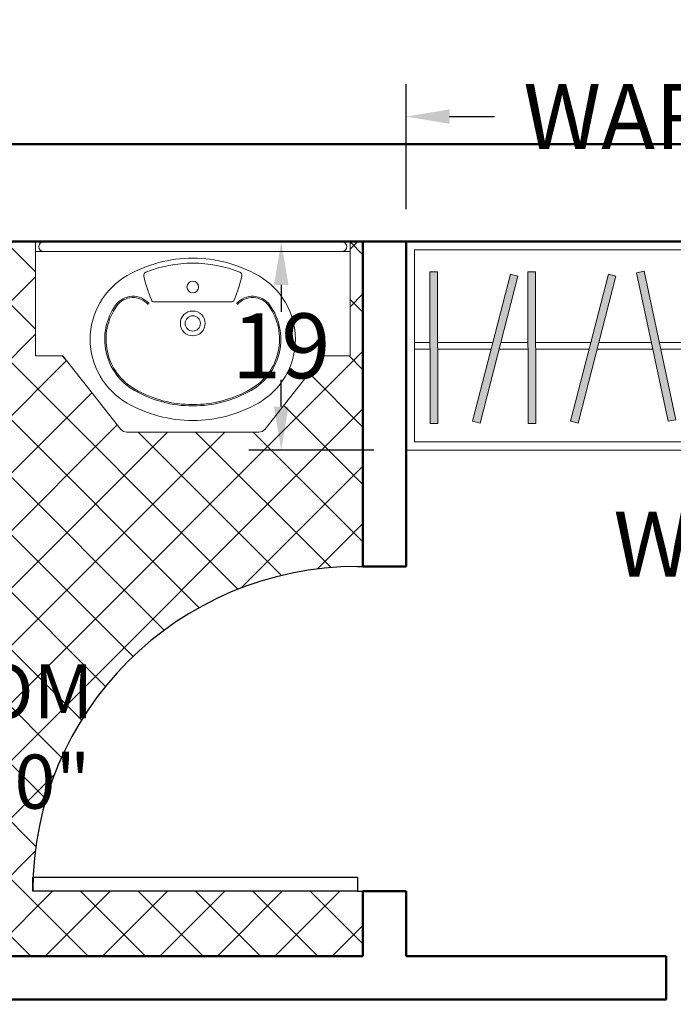
# Model space of a CAD drawing. Units: inches. Extents: x -466983 to 1020, y 324 to 318697.
# Tile 97 of 97: x 870 to 930, y 1006 to 1096. Entities that reach past the tile are written whole.
import ezdxf

# ---------------------------------------------------------------- set-up
doc = ezdxf.new("R2010")
doc.units = ezdxf.units.IN
doc.header["$MEASUREMENT"] = 0
for name, color, linetype, lineweight in [('A-ANNO-DIMS', 2, 'Continuous', 18), ('A-ANNO-TEXT', 7, 'Continuous', 18), ('A-AREA-IDEN', 7, 'Continuous', 25), ('A-DOOR', 3, 'Continuous', 25), ('A-FLOR-FIXT', 9, 'Continuous', 18), ('A-FLOR-PATT', 252, 'Continuous', 13), ('A-FURN', 8, 'Continuous', 18), ('A-WALL', 7, 'Continuous', 50)]:
    doc.layers.add(name, color=color, linetype=linetype, lineweight=lineweight)
doc.styles.get("Standard").update_dxf_attribs({"font": 'arial.ttf'})
doc.dimstyles.get("Standard").update_dxf_attribs({"dimtxt": 6, "dimasz": 4, "dimexe": 3, "dimexo": 3, "dimgap": 0.09, "dimtad": 0, "dimtih": 1, "dimtoh": 1, "dimdec": 1, "dimzin": 0, "dimdsep": 46, "dimlunit": 3, "dimtxsty": 'Standard', "dimcen": 0.09, "dimadec": 0, "dimazin": 0, "dimtfac": 1, "dimtdec": 1, "dimtofl": 0, "dimtmove": 0, "dimatfit": 3, "dimfxl": 1, "dimtolj": 1, "dimtzin": 0, "dimarcsym": 0})

# ---------------------------------------------------------------- blocks, each defined once
blk = doc.blocks.new('*U33')
for p, q in [((0, 0), (-1e-16, -5.999999999999999)), ((40, -6e-16), (40, -6))]:
    blk.add_line(p, q)
blk.add_lwpolyline([(0, 0), (5.6e-15, 40), (1.750000000000007, 40), (1.749999999999998, -7e-16)], close=True)
blk.add_arc((0, 0), 40, 0, 90)
blk = doc.blocks.new('B3')
for p, q in [((-450, 0), (-455.7402514854766, -1.1418070123309)), ((450, 0), (455.7402514854766, -1.1418070123309)), ((-463.8581929876745, -9.25974851452338), (-465, -15)), ((-465, -15), (-463.8581929876745, -20.74025148547662)), ((-460.6066017178018, -4.393398282201815), (-463.8581929876745, -9.25974851452338)), ((-463.8581929876745, -20.74025148547662), (-460.6066017178018, -25.60660171779819)), ((-455.7402514854766, -1.1418070123309), (-460.6066017178018, -4.393398282201815)), ((-460.6066017178018, -25.60660171779819), (-455.7402514854766, -28.8581929876691)), ((-455.7402514854766, -28.8581929876691), (-450, -30)), ((455.7402514854766, -28.8581929876691), (450, -30)), ((455.7402514854766, -1.1418070123309), (460.6066017177945, -4.393398282201815)), ((460.6066017177945, -25.60660171779819), (455.7402514854766, -28.8581929876691)), ((460.6066017177945, -4.393398282201815), (463.8581929876672, -9.25974851452338)), ((463.8581929876672, -20.74025148547662), (460.6066017177945, -25.60660171779819)), ((463.8581929876672, -9.25974851452338), (465, -15)), ((465, -15), (463.8581929876672, -20.74025148547662)), ((475, -30), (-475, -30)), ((2.91038e-11, -182.0000000000054), (-115.8117069986983, -182.0000000000054)), ((2.91038e-11, -182.0000000000054), (115.8117069987565, -182.0000000000054))]:
    blk.add_line(p, q)
blk.add_lwpolyline([(199.4833683843535, -575, 0.2017697719241106), (217.3542190239823, -567.482353886593), (392.5, -345), (435, -345), (475, -345), (475, 0), (-475, 0), (-475, -345), (-435, -345), (-392.5, -345), (-217.3542190239896, -567.482353886593, 0.2017697719241107), (-199.4833683843608, -575)], format="xyb", close=True)
for centre, radius, start, end in [((5.09317e-11, -450.0000000000327), 400.0000000000322, 90, 119.7172288959075), ((0, -450.0000000000327), 400.0000000000319, 60.28277110409252, 90), ((2.91038e-11, -450.0000000000055), 385, 90, 111.6513567404431), ((2.91038e-11, -450.0000000000055), 385, 68.34864325955687, 90), ((-88.47222222221171, -295.0000000000055), 221.527777777762, 119.7172288959075, 240.2827711040925), ((-138.3591766736499, -101.4576952073475), 10, 111.6513567404431, 193.3915177581575), ((338.3178096717893, 12.0282100348104), 500, 193.3915177581575, 202.0594091764406), ((-338.3178096717383, 12.0282100348104), 500, 337.9405908235594, 346.6084822418425), ((138.3591766737008, -101.4576952073475), 10, 346.6084822418425, 68.34864325955687), ((88.47222222225537, -294.9999999999964), 221.527777777762, 299.7172288959074, 60.28277110409252), ((2.91038e-11, -136.9999999999891), 17.5, 90, 270), ((2.91038e-11, -136.9999999999891), 17.5, 270, 90), ((-180.5137974189128, -229.2550553338115), 64.41699441097052, 40.71477974361456, 144.4619255202982), ((-180.5137974189128, -229.2550553338115), 60.41699441097051, 40.71477974361456, 144.4619255202982), ((-115.8117069986983, -172.0000000000145), 10, 202.0594091764406, 270), ((115.8117069987565, -172.0000000000145), 10, 270, 337.9405908235594), ((180.5137974189638, -229.2550553338115), 64.41699441097052, 35.53807447970174, 139.2852202563854), ((180.5137974189638, -229.2550553338115), 60.41699441097051, 35.53807447970174, 139.2852202563854), ((-88.47222222221171, -295.0000000000055), 177.5277777777778, 144.4619255202982, 240.2827711040925), ((-88.47222222221171, -295.0000000000055), 173.5277777777778, 144.4619255202982, 240.2827711040925), ((88.47222222223354, -295.0000000000055), 173.5277777777778, 299.7172288959074, 35.53807447970174), ((88.47222222223354, -295.0000000000055), 177.5277777777778, 299.7172288959074, 35.53807447970174), ((2.91038e-11, -247.0000000000037), 37.5, 90, 270), ((2.91038e-11, -247.0000000000037), 23, 90, 270), ((2.91038e-11, -247.0000000000037), 37.5, 270, 90), ((2.91038e-11, -247.0000000000037), 23, 270, 90), ((2.91038e-11, -140.0000000000036), 352, 240.2827711040925, 270), ((2.91038e-11, -140.0000000000036), 352, 270, 299.7172288959074), ((2.91038e-11, -140.0000000000036), 356, 240.2827711040925, 270), ((2.91038e-11, -140.0000000000036), 356, 270, 299.7172288959074), ((5.09317e-11, -139.9999999999781), 400.0000000000309, 240.2827711040925, 270), ((-1.45519e-11, -140.0000000000309), 399.9999999999781, 270, 299.7172288959074)]:
    blk.add_arc(centre, radius, start, end)
blk = doc.blocks.new('Wardrobe 1.1')
h = blk.add_hatch(color=256)
h.dxf.hatch_style = 1
h.paths.add_polyline_path([(4623.63130591675, 1559.127828082639), (4605.452274823494, 1555.618178042687), (4674.43862754123, 1198.026895294012), (4692.617658634486, 1201.536545333964)])
h = blk.add_hatch(color=256)
h.dxf.hatch_style = 1
h.paths.add_polyline_path([(4989.37316691601, 1559.911022331437), (4970.858516418657, 1559.860704815934), (4971.798831744867, 1195.677017418713), (4990.313482242336, 1195.727334934216)])
h = blk.add_hatch(color=256)
h.dxf.hatch_style = 1
h.paths.add_polyline_path([(3151.282105115228, 1187.510288244974), (3169.796885531561, 1187.510288244974), (3168.856570205235, 1551.693975642194), (3150.341919707882, 1551.643658126692)])
h = blk.add_hatch(color=256)
h.dxf.hatch_style = 1
h.paths.add_polyline_path([(3361.868584936534, 1541.669378461711), (3343.939726713163, 1546.290077294676), (3253.002619132332, 1193.641406768397), (3270.931477355587, 1189.02070793549)])
h = blk.add_hatch(color=256)
h.dxf.hatch_style = 1
h.paths.add_polyline_path([(3403.891248248334, 1551.693975642194), (3385.376597750981, 1551.643658126692), (3386.316913077191, 1187.459970729471), (3404.831563574544, 1187.510288244974)])
h = blk.add_hatch(color=256)
h.dxf.hatch_style = 1
h.paths.add_polyline_path([(3596.9032629794, 1541.669378461711), (3578.974404756262, 1546.290077294676), (3488.037297175316, 1193.641406768397), (3505.966155398454, 1189.02070793549)])
h = blk.add_hatch(color=256)
h.dxf.hatch_style = 1
h.paths.add_polyline_path([(3664.213577620618, 1553.074679382599), (3646.111361609239, 1549.18821693327), (3722.509827192224, 1193.106882382172), (3740.612043203603, 1196.993344831501)])
h = blk.add_hatch(color=256)
h.dxf.hatch_style = 1
h.paths.add_polyline_path([(3813.833679657712, 1190.320201264565), (3832.296488257873, 1188.934736184298), (3859.597907476409, 1552.094859088468), (3841.135098876248, 1553.480324168735)])
h = blk.add_hatch(color=256)
h.dxf.hatch_style = 1
h.paths.add_polyline_path([(4029.392729275909, 1551.693975642194), (4010.878078778556, 1551.643658126692), (4011.818394104767, 1187.459970729471), (4030.333044602236, 1187.510288244974)])
h = blk.add_hatch(color=256)
h.dxf.hatch_style = 1
h.paths.add_polyline_path([(4222.404744007092, 1541.669378461711), (4204.475885783836, 1546.290077294676), (4113.538778203007, 1193.641406768397), (4131.467636426145, 1189.02070793549)])
h = blk.add_hatch(color=256)
h.dxf.hatch_style = 1
h.paths.add_polyline_path([(4348.011308219915, 1193.106882382172), (4366.113524231294, 1196.993344831501), (4289.715058648309, 1553.074679382599), (4271.612842636931, 1549.18821693327)])
h = blk.add_hatch(color=256)
h.dxf.hatch_style = 1
h.paths.add_polyline_path([(4837.600952654661, 1550.260731044678), (4819.316543353771, 1553.17194924514), (4762.004005428219, 1193.525017719703), (4780.288414729109, 1190.613799519242)])
h = blk.add_hatch(color=256)
h.dxf.hatch_style = 1
h.paths.add_polyline_path([(4895.873954488479, 1554.659198605851), (4877.410424046501, 1553.283386659738), (4902.671188982951, 1196.772307061869), (4921.13471942493, 1198.148119007923)])
at = {"ltscale": 5}
for p, q in [((3093.82979383441, 1124.111993690416), (3093.82979383441, 1624.111993690416)), ((3093.82979383441, 1624.111993690416), (5093.829793834409, 1624.111993690416)), ((5093.829793834409, 1624.111993690416), (5093.829793834409, 1124.111993690416)), ((5093.829793834409, 1124.111993690416), (3093.82979383441, 1124.111993690416))]:
    blk.add_line(p, q, dxfattribs=at)
for p, q in [((3113.82979383441, 1144.111993690416), (3113.82979383441, 1604.111993690416)), ((3113.82979383441, 1604.111993690416), (5073.829793834409, 1604.111993690416)), ((5073.829793834409, 1604.111993690416), (5073.829793834409, 1144.111993690416)), ((4623.63130591675, 1559.127828082639), (4605.452274823494, 1555.618178042687)), ((4692.617658634486, 1201.536545333964), (4623.63130591675, 1559.127828082639)), ((4989.37316691601, 1559.911022331437), (4970.858516418657, 1559.860704815934)), ((4970.858516418657, 1559.860704815934), (4971.798831744867, 1195.677017418713)), ((4990.313482242336, 1195.727334934216), (4989.37316691601, 1559.911022331437)), ((3168.856570205235, 1551.693975642194), (3150.341919707882, 1551.643658126692)), ((3150.341919707882, 1551.643658126692), (3151.282235034092, 1187.459970729471)), ((3169.796885531561, 1187.510288244974), (3168.856570205235, 1551.693975642194)), ((3343.939726713163, 1546.290077294676), (3253.002619132332, 1193.641406768397)), ((3270.931477355587, 1189.02070793549), (3361.868584936534, 1541.669378461711)), ((3361.868584936534, 1541.669378461711), (3343.939726713163, 1546.290077294676)), ((3403.891248248334, 1551.693975642194), (3385.376597750981, 1551.643658126692)), ((3385.376597750981, 1551.643658126692), (3386.316913077191, 1187.459970729471)), ((3404.831563574544, 1187.510288244974), (3403.891248248334, 1551.693975642194)), ((3578.974404756262, 1546.290077294676), (3488.037297175316, 1193.641406768397)), ((3505.966155398454, 1189.02070793549), (3596.9032629794, 1541.669378461711)), ((3596.9032629794, 1541.669378461711), (3578.974404756262, 1546.290077294676)), ((3664.213577620618, 1553.074679382599), (3646.111361609239, 1549.18821693327)), ((3646.111361609239, 1549.18821693327), (3722.509827192224, 1193.106882382172)), ((3740.612043203603, 1196.993344831501), (3664.213577620618, 1553.074679382599)), ((3841.135098876248, 1553.480324168735), (3813.833679657712, 1190.320201264565)), ((3832.296488257873, 1188.934736184298), (3859.597907476409, 1552.094859088468)), ((3859.597907476409, 1552.094859088468), (3841.135098876248, 1553.480324168735)), ((4029.392729275909, 1551.693975642194), (4010.878078778556, 1551.643658126692)), ((4010.878078778556, 1551.643658126692), (4011.818394104767, 1187.459970729471)), ((4030.333044602236, 1187.510288244974), (4029.392729275909, 1551.693975642194)), ((4204.475885783836, 1546.290077294676), (4113.538778203007, 1193.641406768397)), ((4131.467636426145, 1189.02070793549), (4222.404744007092, 1541.669378461711)), ((4222.404744007092, 1541.669378461711), (4204.475885783836, 1546.290077294676)), ((4289.715058648309, 1553.074679382599), (4271.612842636931, 1549.18821693327)), ((4271.612842636931, 1549.18821693327), (4348.011308219915, 1193.106882382172)), ((4366.113524231294, 1196.993344831501), (4289.715058648309, 1553.074679382599)), ((4605.452274823494, 1555.618178042687), (4674.43862754123, 1198.026895294012)), ((4819.316543353771, 1553.17194924514), (4762.004005428219, 1193.525017719703)), ((4780.288414729109, 1190.613799519242), (4837.600952654661, 1550.260731044678)), ((4837.600952654661, 1550.260731044678), (4819.316543353771, 1553.17194924514)), ((4895.873954488479, 1554.659198605851), (4877.410424046501, 1553.283386659738)), ((4877.410424046501, 1553.283386659738), (4902.671188982951, 1196.772307061869)), ((4921.13471942493, 1198.148119007923), (4895.873954488479, 1554.659198605851)), ((3150.779647227988, 1382.111993690416), (3113.82979383441, 1382.111993690416)), ((3301.603312885615, 1382.111993690416), (3169.294427644258, 1382.111993690416)), ((3301.603312885671, 1382.111993690416), (3169.294427644278, 1382.111993690416)), ((3385.814325271087, 1382.111993690416), (3320.723705409183, 1382.111993690416)), ((3536.63799092866, 1382.111993690416), (3404.329105687303, 1382.111993690416)), ((3536.637990928537, 1382.111993690416), (3404.329105687377, 1382.111993690416)), ((3681.958135513426, 1382.111993690416), (3555.75838345205, 1382.111993690416)), ((3681.958135513406, 1382.111993690416), (3555.758383452127, 1382.111993690416)), ((3828.252080240405, 1382.111993690416), (3700.894205307252, 1382.111993690416)), ((3828.252080240453, 1382.111993690416), (3700.894205307288, 1382.111993690416)), ((4011.315806298681, 1382.111993690416), (3846.819044447374, 1382.111993690416)), ((4162.139471956229, 1382.111993690416), (4029.830586714952, 1382.111993690416)), ((4307.459616541096, 1382.111993690416), (4181.259864479818, 1382.111993690416)), ((4453.753561268143, 1382.111993690416), (4326.395686334979, 1382.111993690416)), ((4638.925011464094, 1382.111993690416), (4472.320525475011, 1382.111993690416)), ((4792.056807955193, 1382.111993690416), (4657.781122696752, 1382.111993690416)), ((4889.538855865531, 1382.111993690416), (4810.805142536459, 1382.111993690416)), ((4971.317460196375, 1382.111993690416), (4908.099870128257, 1382.111993690416)), ((5073.829793834409, 1382.111993690416), (4989.832240612645, 1382.111993690416)), ((3150.820958922443, 1366.111993690417), (3113.82979383441, 1366.111993690416)), ((3297.477411264826, 1366.111993690417), (3169.335739338719, 1366.111993690417)), ((3297.477411264836, 1366.111993690416), (3169.33573933882, 1366.111993690416)), ((3385.855636965543, 1366.111993690416), (3316.597803788389, 1366.111993690416)), ((3532.512089307866, 1366.111993690416), (3404.370417381759, 1366.111993690416)), ((3532.512089307935, 1366.111993690416), (3404.370417381687, 1366.111993690416)), ((3685.390990119154, 1366.111993690416), (3551.632481831255, 1366.111993690417)), ((3685.390990119244, 1366.111993690416), (3551.632481831408, 1366.111993690416)), ((3827.049242483872, 1366.111993690416), (3704.32705991298, 1366.111993690416)), ((3827.049242483967, 1366.111993690416), (3704.327059913011, 1366.111993690416)), ((4011.357117993108, 1366.111993690416), (3845.61620669084, 1366.111993690416)), ((4158.013570335509, 1366.111993690416), (4029.871898409377, 1366.111993690416)), ((4310.892471146819, 1366.111993690416), (4177.133962858983, 1366.111993690416)), ((4452.550723511541, 1366.111993690416), (4329.828540940702, 1366.111993690416)), ((4642.011724414702, 1366.111993690416), (4471.117687718526, 1366.111993690416)), ((4789.507083415918, 1366.111993690416), (4660.867835647359, 1366.111993690416)), ((4890.672543602346, 1366.111993690416), (4808.255417997067, 1366.111993690416)), ((4971.3587718908, 1366.111993690416), (4909.233557865072, 1366.111993690416)), ((5073.829793834409, 1366.111993690416), (4989.873552307186, 1366.111993690416)), ((3169.796885531561, 1187.510288244974), (3151.282105115229, 1187.510288244974)), ((3253.002619132332, 1193.641406768397), (3270.931477355587, 1189.02070793549)), ((3404.831563574544, 1187.510288244974), (3386.316913077191, 1187.459970729471)), ((3488.037297175316, 1193.641406768397), (3505.966155398454, 1189.02070793549)), ((3722.509827192224, 1193.106882382172), (3740.612043203603, 1196.993344831501)), ((3832.296488257873, 1188.934736184298), (3813.833679657712, 1190.320201264565)), ((4030.333044602236, 1187.510288244974), (4011.818394104767, 1187.459970729471)), ((4113.538778203007, 1193.641406768397), (4131.467636426145, 1189.02070793549)), ((4348.011308219915, 1193.106882382172), (4366.113524231294, 1196.993344831501)), ((4674.43862754123, 1198.026895294012), (4692.617658634486, 1201.536545333964)), ((4762.004005428219, 1193.525017719703), (4780.288414729109, 1190.613799519242)), ((4902.671188982951, 1196.772307061869), (4921.13471942493, 1198.148119007923)), ((4971.798831744867, 1195.677017418713), (4990.313482242336, 1195.727334934216)), ((5073.829793834409, 1144.111993690416), (3113.82979383441, 1144.111993690416))]:
    blk.add_line(p, q)
blk.add_lwpolyline([(4439.335160685403, 1190.320201264565), (4466.63657990394, 1553.480324168735), (4485.0993885041, 1552.094859088468), (4457.797969285564, 1188.934736184298), (4439.231005078596, 1188.934736184298)])
blk = doc.blocks.new('*D85')
at = {"layer": 'A-ANNO-DIMS', "color": 0, "lineweight": -2, "transparency": 16777216}
for p, q in [((905.8056775209042, 1078.937732818421), (905.8056775209042, 1090.487732818421)), ((982.805677520904, 1078.937732818421), (982.805677520904, 1090.487732818421)), ((909.805677520904, 1087.487732818421), (913.9496475072615, 1087.487732818421)), ((978.805677520904, 1087.487732818421), (974.6617075345467, 1087.487732818421))]:
    blk.add_line(p, q, dxfattribs=at)
at = {"layer": 'A-ANNO-DIMS', "color": 0, "transparency": 16777216}
for points in [[(909.805677520904, 1088.154399485087), (909.805677520904, 1086.821066151754), (905.8056775209042, 1087.487732818421)], [(978.805677520904, 1088.154399485087), (978.805677520904, 1086.821066151754), (982.805677520904, 1087.487732818421)]]:
    blk.add_solid(points, dxfattribs=at)
at = {"layer": 'Defpoints', "color": 0, "transparency": 16777216}
for p in [(982.805677520904, 1087.487732818421), (905.8056775209042, 1075.937732818421), (982.805677520904, 1075.937732818421)]:
    blk.add_point(p, dxfattribs=at)
at = {"layer": 'A-ANNO-DIMS', "color": 0, "transparency": 16777216, "insert": (944.305677520904, 1087.487732818421), "char_height": 6, "attachment_point": 5}
blk.add_mtext('\\A1;WARDROBE 77', dxfattribs=at)
blk = doc.blocks.new('*D86')
at = {"layer": 'A-ANNO-DIMS', "color": 0, "lineweight": -2, "transparency": 16777216}
for p, q in [((902.8056775209046, 1075.937732818421), (891.2556775209051, 1075.937732818421)), ((894.2556775209052, 1071.937732818421), (894.2556775209052, 1069.466170744751)), ((894.2556775209052, 1060.687732818421), (894.2556775209052, 1063.159294892091)), ((902.8056775209046, 1056.687732818421), (891.2556775209051, 1056.687732818421))]:
    blk.add_line(p, q, dxfattribs=at)
at = {"layer": 'A-ANNO-DIMS', "color": 0, "transparency": 16777216}
for points in [[(893.5890108542384, 1071.937732818421), (894.9223441875718, 1071.937732818421), (894.2556775209052, 1075.937732818421)], [(893.5890108542384, 1060.687732818421), (894.9223441875718, 1060.687732818421), (894.2556775209052, 1056.687732818421)]]:
    blk.add_solid(points, dxfattribs=at)
at = {"layer": 'Defpoints', "color": 0, "transparency": 16777216}
for p in [(894.2556775209052, 1075.937732818421), (905.8056775209045, 1075.937732818421), (905.8056775209045, 1056.687732818421)]:
    blk.add_point(p, dxfattribs=at)
at = {"layer": 'A-ANNO-DIMS', "color": 0, "transparency": 16777216, "insert": (894.2556775209052, 1066.312732818421), "char_height": 6, "attachment_point": 5}
blk.add_mtext('\\A1;19', dxfattribs=at)

msp = doc.modelspace()

# ---------------------------------------------------------------- hatches: boundary and pattern name
at = {"layer": 'A-FLOR-PATT', "transparency": 33554572}
h = msp.add_hatch(dxfattribs=at)
h.set_pattern_fill('ANSI37', color=256, scale=30)
h.set_pattern_definition([(45, (-1212.413693079869, -290.0350025265127), (-2.651650429449553, 2.651650429449553), []), (135, (-1212.413693079869, -290.0350025265127), (-2.651650429449553, -2.651650429449552), [])])
h.paths.add_polyline_path([(901.805677520904, 1075.937732818422), (900.6144036774049, 1075.937732818422), (900.6144036774049, 1065.385628316983), (899.390971271441, 1065.385628316983), (898.0910743401043, 1065.385628316983), (892.8355944880973, 1058.709752245277, -0.2583770168556315), (892.18750428989, 1058.350891982691), (879.9847834232776, 1058.350891982691, -0.2017697719240963), (879.438188978411, 1058.580825279484), (874.0812133730635, 1065.385628316983), (872.7813164417267, 1065.385628316983), (871.5578840357629, 1065.385628316983), (871.5578840357629, 1075.937732818422), (813.8056775209042, 1075.937732818422), (813.8056775209042, 1044.792233318721), (832.3947444543938, 1044.792233318721, -0.3947951267487684), (848.6601780212009, 1028.535584015862), (848.6601780212009, 1009.937732818421), (901.805677520904, 1009.937732818421), (901.805677520904, 1015.937732818421), (901.3056775209042, 1015.937732818421), (871.3056775209039, 1015.937732818421), (871.3056775209039, 1017.250232818421), (871.3344022102003, 1017.250232818421, -0.4014527144963572), (901.3056775209042, 1045.937732818421), (901.805677520904, 1045.937732818421)])
edge = h.paths.add_edge_path(flags=16)
edge.add_line((847.7730719745084, 1068.948588737025), (847.7730719745069, 1073.708823774771))
edge.add_arc((849.2268986539951, 1073.708823774771), 1.453826679487974, 90, 180, ccw=False)
edge.add_line((849.2268986539951, 1075.162650454259), (864.4920787886183, 1075.162650454259))
edge.add_arc((864.4920787886213, 1073.708823774771), 1.453826679487974, 0, 90.00000000012102, ccw=False)
edge.add_line((865.9459054681093, 1073.708823774771), (865.9459054681081, 1069.00351244647))
edge.add_arc((832.6447385074767, 1068.976050591752), 33.30117828385809, -20.61233806670998, 0.04724903539101888, ccw=False)
edge.add_ellipse((856.8594887213083, 1058.479989307073), major_axis=(-2.091e-13, 10.21313242340307), ratio=0.6859192225533502, start_angle=100.00884331843292, end_angle=259.9911566815624, ccw=False)
edge.add_arc((881.0742389351396, 1068.976050591752), 33.30117828385809, 180.0472490354062, 200.6123380667097, ccw=False)
h.paths.add_polyline_path([(853.145578187156, 1066.481532374271), (853.145578187156, 1066.453444752512), (853.1463399851561, 1066.453444752512, 0.4331071439582673), (852.9166149812349, 1066.684892837266), (852.9166149812349, 1066.453444752512), (853.145578187156, 1066.453444752512), (853.145578187156, 1066.481532374489), (853.088019486549, 1066.612171966583, 0.6979386910037918), (852.699540939094, 1066.453444752512), (852.7003027371272, 1066.453444752512), (852.7003027371272, 1066.481532374489), (852.9166149812349, 1067.001204630995), (852.9166149812349, 1066.684892837266, -0.3962543063594317)], flags=0)
h.paths.add_polyline_path([(861.0186747055222, 1066.481532374271), (861.0186747055222, 1066.453444752512), (861.0194365035225, 1066.453444752512, 0.4164039232557909), (860.8023624614146, 1066.684892837265), (860.8023624614146, 1066.453444752512), (861.0186747055222, 1066.453444752512), (861.0186747055222, 1066.481532374489), (860.9671752720659, 1066.605255499379, 0.7133437187663149), (860.5726374574602, 1066.453444752512), (860.5733992554934, 1066.453444752512), (860.5733992554934, 1066.481532374489), (860.8023624614146, 1067.001204630995), (860.8023624614146, 1066.684892837265, -0.3799725304814568)], flags=0)
edge = h.paths.add_edge_path(flags=0)
edge.add_spline(control_points=[(861.1298377106021, 1065.785468371534), (861.4660965533383, 1065.247811229462), (861.613385559155, 1065.016139861057), (861.9832837951076, 1064.373617117607), (862.1924105327118, 1063.944313665492), (862.5613774174725, 1063.039129539609), (862.7212131906668, 1062.56326642291), (862.9865156700853, 1061.578122280975), (863.0919804897928, 1061.068856600952), (863.2452407883674, 1060.031049745086), (863.293035446714, 1059.502522766744), (863.3294736797056, 1058.440879580113), (863.3181170778639, 1057.907777155726), (863.2366033468288, 1056.85179603536), (863.1664466211855, 1056.328931215311), (862.9695120306455, 1055.307951977375), (862.8427353108815, 1054.809852090196), (862.5365466723708, 1053.852219447362), (862.3571373353129, 1053.392702749349), (861.9514237071658, 1052.524888245794), (861.7251255454219, 1052.116609101398), (861.2330086320977, 1051.362239687588), (860.9672044472572, 1051.016170456457), (860.4047960485765, 1050.394909316517), (860.1082220871676, 1050.119734477926), (859.493696255806, 1049.64606200509), (859.1757900615103, 1049.447558762665), (858.5275631429041, 1049.129883644436), (858.197273503909, 1049.010664382187), (857.5314773710529, 1048.851811036626), (857.1959384637446, 1048.812116564677), (856.5249326641573, 1048.811967422545), (856.1893892160524, 1048.851512676201), (855.5235728169741, 1049.010066967686), (855.1932673158994, 1049.129136347874), (854.5449932971788, 1049.446513839261), (854.2270557868354, 1049.644869411481), (853.6124495619564, 1050.118254324803), (853.3158265363004, 1050.393289340464), (852.7533025914207, 1051.014284587242), (852.487431959371, 1051.360227769297), (851.9951668313728, 1052.114363776776), (851.7687869247744, 1052.522535562859), (851.3628973914427, 1053.390157753425), (851.1833939042357, 1053.849589492002), (850.8770077813263, 1054.807077270704), (850.7501277313783, 1055.30511724975), (850.5529806633081, 1056.326003473117), (850.4827147921034, 1056.848835185142), (850.4009803807432, 1057.904777820697), (850.3895122452288, 1058.437874867502), (850.425728471152, 1059.499535178563), (850.4734126571939, 1060.02808465918), (850.6264565107679, 1061.065963770327), (850.7318153592672, 1061.575279204679), (850.9969137893603, 1062.560548677974), (851.1566514873134, 1063.036487374614), (851.525433403113, 1063.94184619004), (851.7344732542367, 1064.371248757046), (852.1056260411488, 1065.016350037675), (852.2544071072941, 1065.250281998093), (852.608154630964, 1065.733465727338)], knot_values=[3.915332106759953, 3.915332106759953, 3.915332106759953, 3.915332106759953, 4.013467662305501, 4.013467662305501, 4.175531746215815, 4.175531746215815, 4.337595830126129, 4.337595830126129, 4.499659914036444, 4.499659914036444, 4.661723997946757, 4.661723997946757, 4.82378808185707, 4.82378808185707, 4.985852165767384, 4.985852165767384, 5.147916249677697, 5.147916249677697, 5.30998033358801, 5.30998033358801, 5.472044417498324, 5.472044417498324, 5.634108501408637, 5.634108501408637, 5.79617258531895, 5.79617258531895, 5.958236669229264, 5.958236669229264, 6.120300753139577, 6.120300753139577, 6.282364837049891, 6.282364837049891, 6.444428920960204, 6.444428920960204, 6.606493004870517, 6.606493004870517, 6.768557088780831, 6.768557088780831, 6.930621172691144, 6.930621172691144, 7.092685256601457, 7.092685256601457, 7.254749340511771, 7.254749340511771, 7.416813424422084, 7.416813424422084, 7.578877508332397, 7.578877508332397, 7.740941592242711, 7.740941592242711, 7.903005676153024, 7.903005676153024, 8.065069760063338, 8.065069760063338, 8.22713384397365, 8.22713384397365, 8.389197927883965, 8.389197927883965, 8.551262011794279, 8.551262011794279, 8.650370494357087, 8.650370494357087, 8.650370494357087, 8.650370494357087], degree=3, periodic=0)
edge.add_line((852.6421178657537, 1065.785468371534), (861.1298377106024, 1065.785468371534))
edge = h.paths.add_edge_path(flags=0)
edge.add_ellipse((856.8495804607978, 1057.743205248224), major_axis=(-3.1e-13, 7.792134415209829), ratio=0.6878610933899516, start_angle=0, end_angle=360)
h.paths.add_polyline_path([(848.8634419841151, 1069.389059844444), (848.863441984139, 1073.960453158315, -0.4142135623709757), (849.9538119937549, 1075.050823167924), (863.765165448898, 1075.050823167924, -0.4142135623721942), (864.8555354585106, 1073.960453158308), (864.8555354584933, 1069.389059844444, -0.3889362887010341), (864.5236837164459, 1069.026979909221, -0.0435607626104464), (849.19529372618, 1069.02697990933, -0.3889362886276668)], flags=0)
h.paths.add_polyline_path([(853.1006153779753, 1068.112209480768, -1), (852.677499999749, 1068.112209480768, -1)], flags=0)
edge = h.paths.add_edge_path(flags=0)
edge.add_ellipse((856.8594887213083, 1057.33782914961), major_axis=(7.74e-14, 2.20702192546696), ratio=0.6571642650458812, start_angle=0, end_angle=360)
h.paths.add_polyline_path([(861.0414774428674, 1068.112209480768, -1), (860.6183620646412, 1068.112209480768, -1)], flags=0)
edge = h.paths.add_edge_path()
edge.add_line((573.9536545579417, 1057.341203598636), (573.9536545579417, 1075.937732818422))
edge.add_line((573.9536545579417, 1075.937732818422), (558.7307922536265, 1075.937732818422))
edge.add_line((558.7307922536265, 1075.937732818422), (558.7307922536265, 1065.385628316983))
edge.add_line((558.7307922536265, 1065.385628316983), (557.5073598476627, 1065.385628316983))
edge.add_line((557.5073598476627, 1065.385628316983), (556.207462916326, 1065.385628316983))
edge.add_line((556.207462916326, 1065.385628316983), (550.9519830643189, 1058.709752245277))
edge.add_arc((550.3038928661116, 1059.115537236419), 0.7646452537275144, 270, 327.94831933647396, ccw=False)
edge.add_line((550.3038928661116, 1058.350891982691), (538.1011719994992, 1058.350891982691))
edge.add_arc((538.1011719994992, 1059.115537236419), 0.7646452537275137, 224.3704013916024, 270, ccw=False)
edge.add_line((537.5545775546327, 1058.580825279484), (532.1976019492852, 1065.385628316983))
edge.add_line((532.1976019492852, 1065.385628316983), (530.8977050179485, 1065.385628316983))
edge.add_line((530.8977050179485, 1065.385628316983), (529.6742726119846, 1065.385628316983))
edge.add_line((529.6742726119846, 1065.385628316983), (529.6742726119846, 1075.937732818422))
edge.add_line((529.6742726119846, 1075.937732818422), (520.8056775209042, 1075.937732818422))
edge.add_line((520.8056775209042, 1075.937732818422), (520.8056775209042, 1045.937732818422))
edge.add_line((520.8056775209042, 1045.937732818422), (521.3056775209044, 1045.937732818422))
edge.add_arc((521.3056775209042, 1015.937732818422), 30.00000000000023, 2.507490703587223, 89.99999999999977, ccw=False)
edge.add_line((551.2769528316082, 1017.250232818422), (551.3056775209045, 1017.250232818422))
edge.add_line((551.3056775209045, 1017.250232818422), (551.3056775209045, 1015.937732818422))
edge.add_line((551.3056775209045, 1015.937732818422), (520.8056775209042, 1015.937732818422))
edge.add_line((520.8056775209042, 1015.937732818422), (520.8056775209042, 1009.937732818421))
edge.add_line((520.8056775209042, 1009.937732818421), (559.1912990237018, 1010.402158339383))
edge.add_arc((559.1912990237018, 1011.855985018871), 1.453826679487974, 180, 270, ccw=False)
edge.add_line((557.7374723442138, 1011.855985018871), (557.7374723442151, 1016.561296347171))
edge.add_arc((591.0386393048469, 1016.58875820189), 33.3011782838587, 159.3876619332891, 180.0472490353913, ccw=False)
edge.add_ellipse((566.8238890910148, 1027.084819486569), major_axis=(-3.171e-13, 10.21313242340307), ratio=0.6859192225533445, start_angle=280.00884331843395, end_angle=439.99115668156304, ccw=False)
edge.add_arc((542.6091388771833, 1016.58875820189), 33.3011782838584, 0.04724903544490644, 20.612338066710322, ccw=False)
edge.add_line((575.9103058378148, 1016.61622005664), (575.910305837816, 1011.855985018871))
edge.add_arc((574.4564791583282, 1011.855985018871), 1.453826679487974, -90, 0, ccw=False)
edge.add_line((574.4564791583282, 1010.402158339383), (608.8056775209044, 1009.937732818421))
edge.add_line((608.8056775209044, 1009.937732818421), (608.8056775209044, 1041.08570985546))
edge.add_line((608.8056775209044, 1041.08570985546), (590.2179319406538, 1041.08570985546))
edge.add_arc((590.7750219589672, 1057.907380652626), 16.83089295601249, 181.9277454211679, 268.1032059320871, ccw=False)
edge = h.paths.add_edge_path()
edge.add_ellipse((494.2443328575609, 583.6203939656394), major_axis=(-2.099e-13, 10.21313242340307), ratio=0.6859192225533391, start_angle=280.0088433184392, end_angle=439.99115668155895, ccw=False)
edge.add_arc((470.0295826437295, 573.1243326809605), 33.30117828385828, 0.047249035653180727, 20.612338066711573, ccw=False)
edge.add_line((503.3307496043607, 573.1517945358311), (503.3307496043621, 568.3915594979414))
edge.add_arc((501.8769229248741, 568.3915594979414), 1.453826679487974, -90, 0, ccw=False)
edge.add_line((501.8769229248741, 566.9377328184536), (539.8056775209043, 566.9377328184218))
edge.add_line((539.8056775209043, 566.9377328184218), (539.8056775209043, 572.9377328184218))
edge.add_line((539.8056775209043, 572.9377328184218), (539.3056775209043, 572.9377328184218))
edge.add_line((539.3056775209043, 572.9377328184218), (509.3056775209042, 572.9377328184218))
edge.add_line((509.3056775209042, 572.9377328184218), (509.3056775209042, 574.2502328184218))
edge.add_line((509.3056775209042, 574.2502328184218), (509.3344022102004, 574.2502328184218))
edge.add_arc((539.3056775209043, 572.9377328184218), 30.00000000000003, 90, 177.4925092964128, ccw=False)
edge.add_line((539.3056775209043, 602.9377328184218), (539.8056775209043, 602.9377328184218))
edge.add_line((539.8056775209043, 602.9377328184218), (539.8056775209043, 626.9377328184219))
edge.add_line((539.8056775209043, 626.9377328184219), (531.7718318056131, 626.9377328184219))
edge.add_line((531.7718318056131, 626.9377328184219), (531.7718318056131, 616.3856283169836))
edge.add_line((531.7718318056131, 616.3856283169836), (530.5483993996492, 616.3856283169836))
edge.add_line((530.5483993996492, 616.3856283169836), (529.2485024683125, 616.3856283169836))
edge.add_line((529.2485024683125, 616.3856283169836), (523.7105154427977, 609.3508919826913))
edge.add_line((523.7105154427977, 609.3508919826913), (510.7766285267865, 609.3508919826913))
edge.add_line((510.7766285267865, 609.3508919826913), (505.2386415012717, 616.3856283169835))
edge.add_line((505.2386415012717, 616.3856283169835), (503.9387445699351, 616.3856283169836))
edge.add_line((503.9387445699351, 616.3856283169836), (502.7153121639711, 616.3856283169836))
edge.add_line((502.7153121639711, 616.3856283169836), (502.7153121639712, 626.9377328184219))
edge.add_line((502.7153121639712, 626.9377328184219), (481.698294634846, 626.937732818422))
edge.add_line((481.698294634846, 626.937732818422), (481.6982946348461, 610.9950036909872))
edge.add_arc((467.2703297247223, 611.4728203914133), 14.43587476556121, 271.9277454211847, 358.103205932099, ccw=False)
edge.add_line((467.7559403853078, 597.0451157044822), (451.8056775209041, 597.0451157044822))
edge.add_line((451.8056775209041, 597.0451157044822), (451.8056775209041, 584.4035114605515))
edge.add_line((451.8056775209041, 584.4035114605515), (451.8056775209043, 566.9377328184218))
edge.add_line((451.8056775209043, 566.9377328184218), (486.6117427902477, 566.9377328184536))
edge.add_arc((486.6117427902477, 568.3915594979414), 1.453826679487974, 180, 270, ccw=False)
edge.add_line((485.1579161107598, 568.3915594979414), (485.157916110761, 573.0968708261933))
edge.add_arc((518.4590830713927, 573.1243326809608), 33.3011782838585, 159.387661933289, 180.0472490354759, ccw=False)
h.paths.add_polyline_path([(836.2608886421394, 1020.732838196592), (879.8898108795202, 1020.732838196592), (879.8898108795202, 1039.390182443977), (836.2608886421394, 1039.390182443977)], flags=25)
h.paths.add_polyline_path([(549.9851009445293, 1036.749159167106), (593.6140231819099, 1036.749159167106), (593.6140231819099, 1055.406503414491), (549.9851009445293, 1055.406503414491)], flags=24)
h.paths.add_polyline_path([(475.1230325221868, 595.5958681380167), (518.7519547595675, 595.5958681380167), (518.7519547595675, 614.2532123854019), (475.1230325221868, 614.2532123854019)], flags=24)

# ---------------------------------------------------------------- linework, layer by layer
at = {"layer": 'A-WALL'}
for p, q in [((391.8056775209043, 1084.937732818421), (991.8056775209043, 1084.937732818421)), ((813.8056775209042, 1075.937732818422), (982.805677520904, 1075.937732818422)), ((901.805677520904, 1075.937732818422), (901.805677520904, 1045.937732818421)), ((905.8056775209042, 1075.937732818422), (905.8056775209042, 1045.937732818421)), ((905.8056775209042, 1045.937732818421), (901.805677520904, 1045.937732818421)), ((905.8056775209042, 1015.937732818421), (901.805677520904, 1015.937732818421)), ((901.805677520904, 1015.937732818421), (901.805677520904, 1009.937732818421)), ((905.8056775209042, 1015.937732818421), (905.8056775209042, 1009.937732818421)), ((901.805677520904, 1009.937732818421), (813.8056775209042, 1009.937732818421)), ((929.8056775209042, 1009.937732818421), (905.8056775209042, 1009.937732818421)), ((929.805677520904, 1009.937732818421), (929.8056775209042, 1005.937732818421)), ((929.8056775209042, 1005.937732818421), (813.8056775209042, 1005.937732818422))]:
    msp.add_line(p, q, dxfattribs=at)

# ---------------------------------------------------------------- block references
at = {"layer": 'A-DOOR', "xscale": 0.7500000000000061, "yscale": 0.7500000000000061, "zscale": 0.7500000000000061, "rotation": 90}
msp.add_blockref('*U33', (901.3056775209042, 1015.937732818421), dxfattribs=at)
at = {"layer": 'A-FLOR-FIXT', "xscale": 0.0305858101490967, "yscale": 0.0305858101490967, "zscale": 0.0305858101490967}
msp.add_blockref('B3', (886.0861438565839, 1075.937732818422), dxfattribs=at)
at = {"layer": 'A-FURN', "xscale": 0.0385, "yscale": 0.0385, "zscale": 0.0385}
msp.add_blockref('Wardrobe 1.1', (786.6932304582793, 1013.40942106134), dxfattribs=at)

# ---------------------------------------------------------------- texts
at = {"layer": 'A-ANNO-TEXT', "insert": (832.3947444543959, 1051.000964560194), "char_height": 6, "attachment_point": 1}
msp.add_mtext_dynamic_manual_height_columns('\\pxqc;WARDROBE', width=229.5582916082931, gutter_width=1, heights=[0], dxfattribs=at)
at = {"layer": 'A-AREA-IDEN', "insert": (823.1222914307581, 1036.902119688179), "char_height": 5, "attachment_point": 1}
msp.add_mtext_dynamic_manual_height_columns('\\pxqc;{\\fArial|b1|i0|c0|p34;BATHROOM\\P7\'-4" X 5\'-0"}', width=69.92316986614605, gutter_width=1, heights=[0], dxfattribs=at)

# ---------------------------------------------------------------- dimensions: what is measured, and where the dimension line sits
at = {"layer": 'A-ANNO-DIMS'}
dim = msp.add_linear_dim(base=(982.805677520904, 1087.487732818421), p1=(905.8056775209042, 1075.937732818421), p2=(982.805677520904, 1075.937732818421), text='WARDROBE <>', dimstyle='Standard', override={"dimdec": 0, "dimlfac": 1, "dimrnd": 0, "dimzin": 0, "dimdsep": 46, "dimlunit": 2}, dxfattribs=at)
dim.commit()
dim.dimension.update_dxf_attribs({"geometry": '*D85', "text_midpoint": (944.305677520904, 1087.487732818421)})
dim = msp.add_linear_dim(base=(894.2556775209052, 1075.937732818421), p1=(905.8056775209042, 1056.687732818421), p2=(905.8056775209042, 1075.937732818421), angle=90, dimstyle='Standard', override={"dimdec": 0, "dimlfac": 1, "dimrnd": 0, "dimzin": 0, "dimdsep": 46, "dimlunit": 2}, dxfattribs=at)
dim.commit()
dim.dimension.update_dxf_attribs({"geometry": '*D86', "text_midpoint": (894.2556775209052, 1066.312732818421)})

doc.saveas('drawing.dxf')
